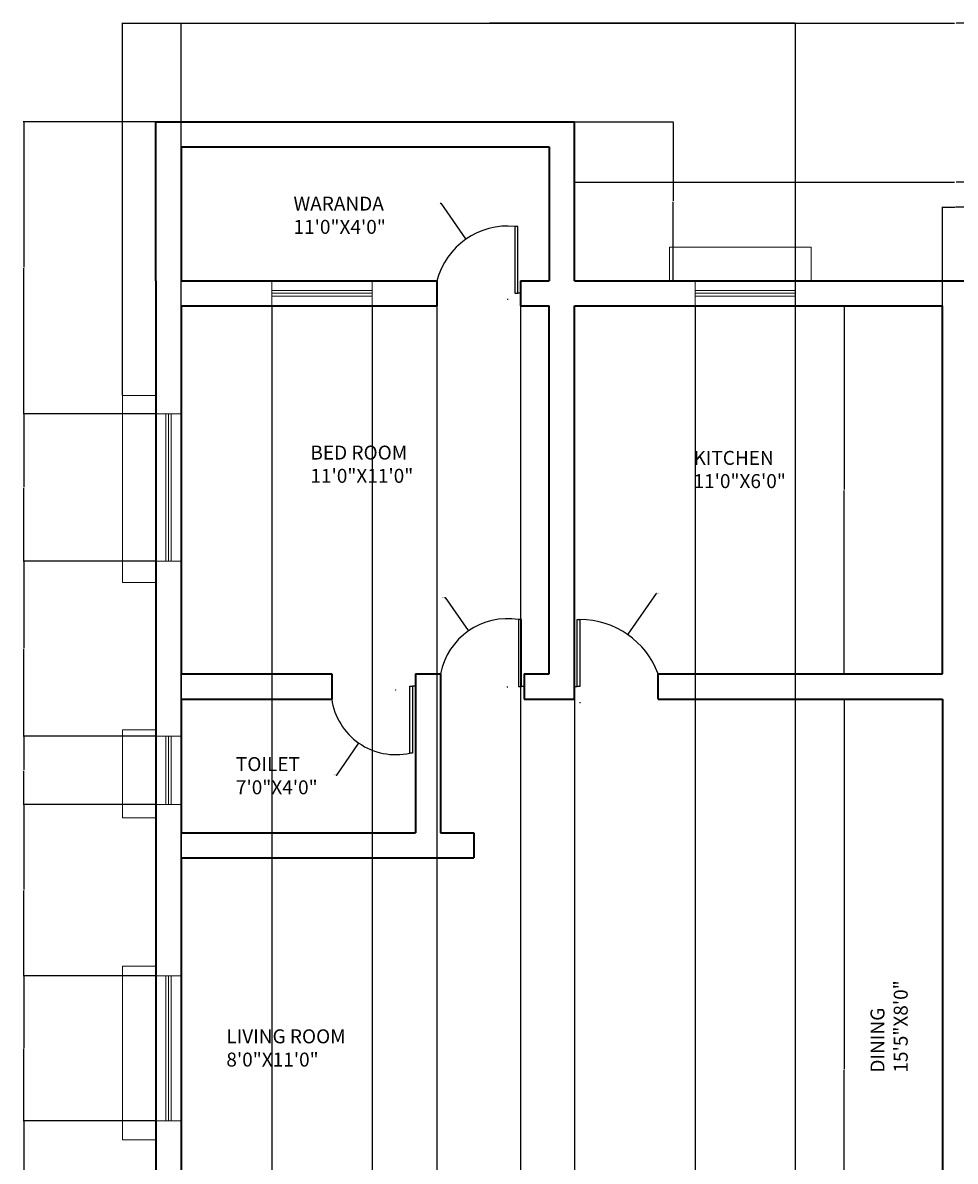
# Model space of a CAD drawing. Units: inches. Extents: x -35 to 633, y -653 to 119.
# Tile 3 of 4: x -35 to 299, y -289 to 119. Entities that reach past the tile are written whole.
import ezdxf

# ---------------------------------------------------------------- set-up
doc = ezdxf.new("R2010")
doc.units = ezdxf.units.IN
doc.header["$MEASUREMENT"] = 0
for name, color, linetype, lineweight in [('A-ANNO-DIMS', 2, 'Continuous', 18), ('A-AREA-IDEN', 7, 'Continuous', 18), ('A-DOOR', 3, 'Continuous', 25), ('A-GLAZ', 4, 'Continuous', 20), ('A-GLAZ-PROJ', 4, 'Continuous', 18), ('A-WALL', 7, 'Continuous', 35)]:
    doc.layers.add(name, color=color, linetype=linetype, lineweight=lineweight)
doc.styles.get("Standard").update_dxf_attribs({"font": 'arial.ttf'})
doc.dimstyles.get("Standard").update_dxf_attribs({"dimtxt": 0.18, "dimasz": 0.18, "dimexe": 0.18, "dimexo": 0.0625, "dimgap": 0.09, "dimtad": 0, "dimtih": 1, "dimtoh": 1, "dimdec": 4, "dimzin": 0, "dimdsep": 46, "dimtxsty": 'Standard', "dimcen": 0.09, "dimadec": 0, "dimazin": 0, "dimtfac": 1, "dimtdec": 4, "dimtofl": 0, "dimtmove": 0, "dimatfit": 3, "dimfxl": 1, "dimtolj": 1, "dimtzin": 0, "dimarcsym": 0})

# ---------------------------------------------------------------- blocks, each defined once
blk = doc.blocks.new('DOOR-LEAF-24IN')
for p, q in [((-1, 24), (-2, 24)), ((-2, 24), (-2, 0)), ((-1, 0), (-1, 24)), ((-2, 0), (-1, 0)), ((0, 0), (-1, 0))]:
    blk.add_line(p, q)
blk = doc.blocks.new('*D11')
at = {"layer": 'A-ANNO-DIMS', "color": 0, "lineweight": -2, "transparency": 16777216}
for p, q in [((0.69, -14.75), (0.69, 118.82)), ((0.87, 118.64), (298.9, 118.64)), ((597.51, 118.64), (299.48, 118.64)), ((597.69, -17.48), (597.69, 118.82))]:
    blk.add_line(p, q, dxfattribs=at)
at = {"layer": 'A-ANNO-DIMS', "color": 0, "transparency": 16777216}
for points in [[(0.87, 118.67), (0.87, 118.61), (0.69, 118.64)], [(597.51, 118.67), (597.51, 118.61), (597.69, 118.64)]]:
    blk.add_solid(points, dxfattribs=at)
at = {"layer": 'Defpoints', "color": 0, "transparency": 16777216}
for p in [(597.69, 118.64), (0.69, -14.81), (597.69, -17.55)]:
    blk.add_point(p, dxfattribs=at)
at = {"layer": 'A-ANNO-DIMS', "color": 0, "transparency": 16777216, "insert": (299.19, 118.64), "char_height": 0.18, "attachment_point": 5}
blk.add_mtext('\\A1;597', dxfattribs=at)
blk = doc.blocks.new('*D12')
at = {"layer": 'A-ANNO-DIMS', "color": 0, "lineweight": -2, "transparency": 16777216}
for p, q in [((162.69, 26.35), (162.69, 61.82)), ((162.87, 61.64), (298.9, 61.64)), ((435.51, 61.64), (299.48, 61.64)), ((435.69, 26.35), (435.69, 61.82))]:
    blk.add_line(p, q, dxfattribs=at)
at = {"layer": 'A-ANNO-DIMS', "color": 0, "transparency": 16777216}
for points in [[(162.87, 61.67), (162.87, 61.61), (162.69, 61.64)], [(435.51, 61.67), (435.51, 61.61), (435.69, 61.64)]]:
    blk.add_solid(points, dxfattribs=at)
at = {"layer": 'Defpoints', "color": 0, "transparency": 16777216}
for p in [(435.69, 61.64), (162.69, 26.29), (435.69, 26.29)]:
    blk.add_point(p, dxfattribs=at)
at = {"layer": 'A-ANNO-DIMS', "color": 0, "transparency": 16777216, "insert": (299.19, 61.64), "char_height": 0.18, "attachment_point": 5}
blk.add_mtext('\\A1;273', dxfattribs=at)
blk = doc.blocks.new('*D13')
at = {"layer": 'A-ANNO-DIMS', "color": 0, "lineweight": -2, "transparency": 16777216}
for p, q in [((162.75, 83.29), (198.22, 83.29)), ((198.04, 83.11), (198.04, 54.97)), ((198.04, 26.47), (198.04, 54.61)), ((162.75, 26.29), (198.22, 26.29))]:
    blk.add_line(p, q, dxfattribs=at)
at = {"layer": 'A-ANNO-DIMS', "color": 0, "transparency": 16777216}
for points in [[(198.01, 83.11), (198.07, 83.11), (198.04, 83.29)], [(198.01, 26.47), (198.07, 26.47), (198.04, 26.29)]]:
    blk.add_solid(points, dxfattribs=at)
at = {"layer": 'Defpoints', "color": 0, "transparency": 16777216}
for p in [(162.69, 83.29), (162.69, 26.29), (198.04, 26.29)]:
    blk.add_point(p, dxfattribs=at)
at = {"layer": 'A-ANNO-DIMS', "color": 0, "transparency": 16777216, "insert": (198.04, 54.79), "char_height": 0.18, "attachment_point": 5}
blk.add_mtext('\\A1;57', dxfattribs=at)
blk = doc.blocks.new('*D14')
at = {"layer": 'A-ANNO-DIMS', "color": 0, "lineweight": -2, "transparency": 16777216}
for p, q in [((21.69, 17.22), (21.69, -652.72)), ((54.19, 17.22), (54.19, -652.72)), ((21.87, -652.54), (37.47, -652.54)), ((54.01, -652.54), (38.4, -652.54))]:
    blk.add_line(p, q, dxfattribs=at)
at = {"layer": 'A-ANNO-DIMS', "color": 0, "transparency": 16777216}
for points in [[(21.87, -652.51), (21.87, -652.57), (21.69, -652.54)], [(54.01, -652.51), (54.01, -652.57), (54.19, -652.54)]]:
    blk.add_solid(points, dxfattribs=at)
at = {"layer": 'Defpoints', "color": 0, "transparency": 16777216}
for p in [(21.69, 17.29), (54.19, 17.29), (54.19, -652.54)]:
    blk.add_point(p, dxfattribs=at)
at = {"layer": 'A-ANNO-DIMS', "color": 0, "transparency": 16777216, "insert": (37.94, -652.54), "char_height": 0.18, "attachment_point": 5}
blk.add_mtext('\\A1;32.496', dxfattribs=at)
blk = doc.blocks.new('*D15')
at = {"layer": 'A-ANNO-DIMS', "color": 0, "lineweight": -2, "transparency": 16777216}
for p, q in [((90.19, 17.22), (90.19, -652.72)), ((113.38, 17.22), (113.38, -652.72)), ((90.37, -652.54), (101.32, -652.54)), ((113.2, -652.54), (102.25, -652.54))]:
    blk.add_line(p, q, dxfattribs=at)
at = {"layer": 'A-ANNO-DIMS', "color": 0, "transparency": 16777216}
for points in [[(90.37, -652.51), (90.37, -652.57), (90.19, -652.54)], [(113.2, -652.51), (113.2, -652.57), (113.38, -652.54)]]:
    blk.add_solid(points, dxfattribs=at)
at = {"layer": 'Defpoints', "color": 0, "transparency": 16777216}
for p in [(90.19, 17.29), (113.38, 17.29), (113.38, -652.54)]:
    blk.add_point(p, dxfattribs=at)
at = {"layer": 'A-ANNO-DIMS', "color": 0, "transparency": 16777216, "insert": (101.78, -652.54), "char_height": 0.18, "attachment_point": 5}
blk.add_mtext('\\A1;23.194', dxfattribs=at)
blk = doc.blocks.new('*D16')
at = {"layer": 'A-ANNO-DIMS', "color": 0, "lineweight": -2, "transparency": 16777216}
for p, q in [((113.38, 17.22), (113.38, -652.72)), ((143.38, 17.22), (143.38, -652.72)), ((113.56, -652.54), (128.16, -652.54)), ((143.2, -652.54), (128.6, -652.54))]:
    blk.add_line(p, q, dxfattribs=at)
at = {"layer": 'A-ANNO-DIMS', "color": 0, "transparency": 16777216}
for points in [[(113.56, -652.51), (113.56, -652.57), (113.38, -652.54)], [(143.2, -652.51), (143.2, -652.57), (143.38, -652.54)]]:
    blk.add_solid(points, dxfattribs=at)
at = {"layer": 'Defpoints', "color": 0, "transparency": 16777216}
for p in [(113.38, 17.29), (143.38, 17.29), (143.38, -652.54)]:
    blk.add_point(p, dxfattribs=at)
at = {"layer": 'A-ANNO-DIMS', "color": 0, "transparency": 16777216, "insert": (128.38, -652.54), "char_height": 0.18, "attachment_point": 5}
blk.add_mtext('\\A1;30', dxfattribs=at)
blk = doc.blocks.new('*D17')
at = {"layer": 'A-ANNO-DIMS', "color": 0, "lineweight": -2, "transparency": 16777216}
for p, q in [((162.69, 17.22), (162.69, -652.72)), ((205.96, 17.22), (205.96, -652.72)), ((162.87, -652.54), (183.93, -652.54)), ((205.78, -652.54), (184.72, -652.54))]:
    blk.add_line(p, q, dxfattribs=at)
at = {"layer": 'A-ANNO-DIMS', "color": 0, "transparency": 16777216}
for points in [[(162.87, -652.51), (162.87, -652.57), (162.69, -652.54)], [(205.78, -652.51), (205.78, -652.57), (205.96, -652.54)]]:
    blk.add_solid(points, dxfattribs=at)
at = {"layer": 'Defpoints', "color": 0, "transparency": 16777216}
for p in [(162.69, 17.29), (205.96, 17.29), (205.96, -652.54)]:
    blk.add_point(p, dxfattribs=at)
at = {"layer": 'A-ANNO-DIMS', "color": 0, "transparency": 16777216, "insert": (184.33, -652.54), "char_height": 0.18, "attachment_point": 5}
blk.add_mtext('\\A1;43.27', dxfattribs=at)
blk = doc.blocks.new('*D18')
at = {"layer": 'A-ANNO-DIMS', "color": 0, "lineweight": -2, "transparency": 16777216}
for p, q in [((294.69, 17.35), (294.69, 52.82)), ((294.87, 52.64), (299.04, 52.64)), ((303.51, 52.64), (299.34, 52.64)), ((303.69, 17.35), (303.69, 52.82))]:
    blk.add_line(p, q, dxfattribs=at)
at = {"layer": 'A-ANNO-DIMS', "color": 0, "transparency": 16777216}
for points in [[(294.87, 52.67), (294.87, 52.61), (294.69, 52.64)], [(303.51, 52.67), (303.51, 52.61), (303.69, 52.64)]]:
    blk.add_solid(points, dxfattribs=at)
at = {"layer": 'Defpoints', "color": 0, "transparency": 16777216}
for p in [(303.69, 52.64), (294.69, 17.29), (303.69, 17.29)]:
    blk.add_point(p, dxfattribs=at)
at = {"layer": 'A-ANNO-DIMS', "color": 0, "transparency": 16777216, "insert": (299.19, 52.64), "char_height": 0.18, "attachment_point": 5}
blk.add_mtext('\\A1;9', dxfattribs=at)
blk = doc.blocks.new('*D25')
at = {"layer": 'A-ANNO-DIMS', "color": 0, "lineweight": -2, "transparency": 16777216}
for p, q in [((12.63, 83.29), (-34.84, 83.29)), ((-34.66, 83.11), (-34.66, 31.12)), ((-34.66, -21.23), (-34.66, 30.76)), ((12.63, -21.41), (-34.84, -21.41))]:
    blk.add_line(p, q, dxfattribs=at)
at = {"layer": 'A-ANNO-DIMS', "color": 0, "transparency": 16777216}
for points in [[(-34.69, 83.11), (-34.63, 83.11), (-34.66, 83.29)], [(-34.69, -21.23), (-34.63, -21.23), (-34.66, -21.41)]]:
    blk.add_solid(points, dxfattribs=at)
at = {"layer": 'Defpoints', "color": 0, "transparency": 16777216}
for p in [(12.69, 83.29), (-34.66, -21.41), (12.69, -21.41)]:
    blk.add_point(p, dxfattribs=at)
at = {"layer": 'A-ANNO-DIMS', "color": 0, "transparency": 16777216, "insert": (-34.66, 30.94), "char_height": 0.18, "attachment_point": 5}
blk.add_mtext('\\A1;104.7', dxfattribs=at)
blk = doc.blocks.new('*D26')
at = {"layer": 'A-ANNO-DIMS', "color": 0, "lineweight": -2, "transparency": 16777216}
for p, q in [((12.63, -21.41), (-34.84, -21.41)), ((-34.66, -21.59), (-34.66, -47.65)), ((-34.66, -74.08), (-34.66, -48.02)), ((12.63, -74.26), (-34.84, -74.26))]:
    blk.add_line(p, q, dxfattribs=at)
at = {"layer": 'A-ANNO-DIMS', "color": 0, "transparency": 16777216}
for points in [[(-34.69, -21.59), (-34.63, -21.59), (-34.66, -21.41)], [(-34.69, -74.08), (-34.63, -74.08), (-34.66, -74.26)]]:
    blk.add_solid(points, dxfattribs=at)
at = {"layer": 'Defpoints', "color": 0, "transparency": 16777216}
for p in [(12.69, -21.41), (-34.66, -74.26), (12.69, -74.26)]:
    blk.add_point(p, dxfattribs=at)
at = {"layer": 'A-ANNO-DIMS', "color": 0, "transparency": 16777216, "insert": (-34.66, -47.84), "char_height": 0.18, "attachment_point": 5}
blk.add_mtext('\\A1;52.85', dxfattribs=at)
blk = doc.blocks.new('*D27')
at = {"layer": 'A-ANNO-DIMS', "color": 0, "lineweight": -2, "transparency": 16777216}
for p, q in [((12.63, -74.26), (-34.84, -74.26)), ((-34.66, -74.44), (-34.66, -105.47)), ((-34.66, -136.87), (-34.66, -105.84)), ((12.63, -137.05), (-34.84, -137.05))]:
    blk.add_line(p, q, dxfattribs=at)
at = {"layer": 'A-ANNO-DIMS', "color": 0, "transparency": 16777216}
for points in [[(-34.69, -74.44), (-34.63, -74.44), (-34.66, -74.26)], [(-34.69, -136.87), (-34.63, -136.87), (-34.66, -137.05)]]:
    blk.add_solid(points, dxfattribs=at)
at = {"layer": 'Defpoints', "color": 0, "transparency": 16777216}
for p in [(12.69, -74.26), (-34.66, -137.05), (12.69, -137.05)]:
    blk.add_point(p, dxfattribs=at)
at = {"layer": 'A-ANNO-DIMS', "color": 0, "transparency": 16777216, "insert": (-34.66, -105.66), "char_height": 0.18, "attachment_point": 5}
blk.add_mtext('\\A1;62.79', dxfattribs=at)
blk = doc.blocks.new('*D28')
at = {"layer": 'A-ANNO-DIMS', "color": 0, "lineweight": -2, "transparency": 16777216}
for p, q in [((12.63, -137.05), (-34.84, -137.05)), ((-34.66, -137.23), (-34.66, -149.1)), ((-34.66, -161.33), (-34.66, -149.46)), ((12.63, -161.51), (-34.84, -161.51))]:
    blk.add_line(p, q, dxfattribs=at)
at = {"layer": 'A-ANNO-DIMS', "color": 0, "transparency": 16777216}
for points in [[(-34.69, -137.23), (-34.63, -137.23), (-34.66, -137.05)], [(-34.69, -161.33), (-34.63, -161.33), (-34.66, -161.51)]]:
    blk.add_solid(points, dxfattribs=at)
at = {"layer": 'Defpoints', "color": 0, "transparency": 16777216}
for p in [(12.69, -137.05), (-34.66, -161.51), (12.69, -161.51)]:
    blk.add_point(p, dxfattribs=at)
at = {"layer": 'A-ANNO-DIMS', "color": 0, "transparency": 16777216, "insert": (-34.66, -149.28), "char_height": 0.18, "attachment_point": 5}
blk.add_mtext('\\A1;24.463', dxfattribs=at)
blk = doc.blocks.new('*D29')
at = {"layer": 'A-ANNO-DIMS', "color": 0, "lineweight": -2, "transparency": 16777216}
for p, q in [((12.63, -161.51), (-34.84, -161.51)), ((-34.66, -161.69), (-34.66, -192.06)), ((-34.66, -222.79), (-34.66, -192.43)), ((12.63, -222.97), (-34.84, -222.97))]:
    blk.add_line(p, q, dxfattribs=at)
at = {"layer": 'A-ANNO-DIMS', "color": 0, "transparency": 16777216}
for points in [[(-34.69, -161.69), (-34.63, -161.69), (-34.66, -161.51)], [(-34.69, -222.79), (-34.63, -222.79), (-34.66, -222.97)]]:
    blk.add_solid(points, dxfattribs=at)
at = {"layer": 'Defpoints', "color": 0, "transparency": 16777216}
for p in [(12.69, -161.51), (-34.66, -222.97), (12.69, -222.97)]:
    blk.add_point(p, dxfattribs=at)
at = {"layer": 'A-ANNO-DIMS', "color": 0, "transparency": 16777216, "insert": (-34.66, -192.24), "char_height": 0.18, "attachment_point": 5}
blk.add_mtext('\\A1;61.46', dxfattribs=at)
blk = doc.blocks.new('*D30')
at = {"layer": 'A-ANNO-DIMS', "color": 0, "lineweight": -2, "transparency": 16777216}
for p, q in [((12.63, -222.97), (-34.84, -222.97)), ((-34.66, -223.15), (-34.66, -248.78)), ((-34.66, -274.78), (-34.66, -249.15)), ((12.63, -274.96), (-34.84, -274.96))]:
    blk.add_line(p, q, dxfattribs=at)
at = {"layer": 'A-ANNO-DIMS', "color": 0, "transparency": 16777216}
for points in [[(-34.69, -223.15), (-34.63, -223.15), (-34.66, -222.97)], [(-34.69, -274.78), (-34.63, -274.78), (-34.66, -274.96)]]:
    blk.add_solid(points, dxfattribs=at)
at = {"layer": 'Defpoints', "color": 0, "transparency": 16777216}
for p in [(12.69, -222.97), (-34.66, -274.96), (12.69, -274.96)]:
    blk.add_point(p, dxfattribs=at)
at = {"layer": 'A-ANNO-DIMS', "color": 0, "transparency": 16777216, "insert": (-34.66, -248.97), "char_height": 0.18, "attachment_point": 5}
blk.add_mtext('\\A1;51.99', dxfattribs=at)
blk = doc.blocks.new('*D31')
at = {"layer": 'A-ANNO-DIMS', "color": 0, "lineweight": -2, "transparency": 16777216}
for p, q in [((12.63, -274.96), (-34.84, -274.96)), ((-34.66, -275.14), (-34.66, -304.9)), ((-34.66, -335.03), (-34.66, -305.27)), ((12.63, -335.21), (-34.84, -335.21))]:
    blk.add_line(p, q, dxfattribs=at)
at = {"layer": 'A-ANNO-DIMS', "color": 0, "transparency": 16777216}
for points in [[(-34.69, -275.14), (-34.63, -275.14), (-34.66, -274.96)], [(-34.69, -335.03), (-34.63, -335.03), (-34.66, -335.21)]]:
    blk.add_solid(points, dxfattribs=at)
at = {"layer": 'Defpoints', "color": 0, "transparency": 16777216}
for p in [(12.69, -274.96), (-34.66, -335.21), (12.69, -335.21)]:
    blk.add_point(p, dxfattribs=at)
at = {"layer": 'A-ANNO-DIMS', "color": 0, "transparency": 16777216, "insert": (-34.66, -305.09), "char_height": 0.18, "attachment_point": 5}
blk.add_mtext('\\A1;60.25', dxfattribs=at)
blk = doc.blocks.new('*D36')
at = {"layer": 'A-ANNO-DIMS', "color": 0, "lineweight": -2, "transparency": 16777216}
for p, q in [((21.69, -546.65), (21.69, 118.82)), ((21.87, 118.64), (131.44, 118.64)), ((241.8, 118.64), (132.23, 118.64)), ((241.98, -546.65), (241.98, 118.82))]:
    blk.add_line(p, q, dxfattribs=at)
at = {"layer": 'A-ANNO-DIMS', "color": 0, "transparency": 16777216}
for points in [[(21.87, 118.67), (21.87, 118.61), (21.69, 118.64)], [(241.8, 118.67), (241.8, 118.61), (241.98, 118.64)]]:
    blk.add_solid(points, dxfattribs=at)
at = {"layer": 'Defpoints', "color": 0, "transparency": 16777216}
for p in [(241.98, 118.64), (21.69, -546.71), (241.98, -546.71)]:
    blk.add_point(p, dxfattribs=at)
at = {"layer": 'A-ANNO-DIMS', "color": 0, "transparency": 16777216, "insert": (131.83, 118.64), "char_height": 0.18, "attachment_point": 5}
blk.add_mtext('\\A1;220.3', dxfattribs=at)
blk = doc.blocks.new('*D38')
at = {"layer": 'A-ANNO-DIMS', "color": 0, "lineweight": -2, "transparency": 16777216}
for p, q in [((294.63, 17.29), (259.16, 17.29)), ((259.34, 17.11), (259.34, -48.53)), ((259.34, -114.53), (259.34, -48.89)), ((294.63, -114.71), (259.16, -114.71))]:
    blk.add_line(p, q, dxfattribs=at)
at = {"layer": 'A-ANNO-DIMS', "color": 0, "transparency": 16777216}
for points in [[(259.31, 17.11), (259.37, 17.11), (259.34, 17.29)], [(259.31, -114.53), (259.37, -114.53), (259.34, -114.71)]]:
    blk.add_solid(points, dxfattribs=at)
at = {"layer": 'Defpoints', "color": 0, "transparency": 16777216}
for p in [(259.34, 17.29), (294.69, 17.29), (294.69, -114.71)]:
    blk.add_point(p, dxfattribs=at)
at = {"layer": 'A-ANNO-DIMS', "color": 0, "transparency": 16777216, "insert": (259.34, -48.71), "char_height": 0.18, "attachment_point": 5}
blk.add_mtext('\\A1;132', dxfattribs=at)
blk = doc.blocks.new('*D46')
at = {"layer": 'A-ANNO-DIMS', "color": 0, "lineweight": -2, "transparency": 16777216}
for p, q in [((294.63, -123.71), (259.16, -123.71)), ((259.34, -123.89), (259.34, -256.48)), ((259.34, -389.42), (259.34, -256.84)), ((294.63, -389.6), (259.16, -389.6))]:
    blk.add_line(p, q, dxfattribs=at)
at = {"layer": 'A-ANNO-DIMS', "color": 0, "transparency": 16777216}
for points in [[(259.31, -123.89), (259.37, -123.89), (259.34, -123.71)], [(259.31, -389.42), (259.37, -389.42), (259.34, -389.6)]]:
    blk.add_solid(points, dxfattribs=at)
at = {"layer": 'Defpoints', "color": 0, "transparency": 16777216}
for p in [(259.34, -123.71), (294.69, -123.71), (294.69, -389.6)]:
    blk.add_point(p, dxfattribs=at)
at = {"layer": 'A-ANNO-DIMS', "color": 0, "transparency": 16777216, "insert": (259.34, -256.66), "char_height": 0.18, "attachment_point": 5}
blk.add_mtext('\\A1;265.9', dxfattribs=at)
blk = doc.blocks.new('*D47')
at = {"layer": 'A-ANNO-DIMS', "color": 0, "lineweight": -2, "transparency": 16777216}
for p, q in [((294.69, -123.78), (294.69, -652.72)), ((126.69, -312.78), (126.69, -652.72)), ((126.87, -652.54), (210.41, -652.54)), ((294.51, -652.54), (210.97, -652.54))]:
    blk.add_line(p, q, dxfattribs=at)
at = {"layer": 'A-ANNO-DIMS', "color": 0, "transparency": 16777216}
for points in [[(126.87, -652.51), (126.87, -652.57), (126.69, -652.54)], [(294.51, -652.51), (294.51, -652.57), (294.69, -652.54)]]:
    blk.add_solid(points, dxfattribs=at)
at = {"layer": 'Defpoints', "color": 0, "transparency": 16777216}
for p in [(294.69, -123.71), (126.69, -312.71), (294.69, -652.54)]:
    blk.add_point(p, dxfattribs=at)
at = {"layer": 'A-ANNO-DIMS', "color": 0, "transparency": 16777216, "insert": (210.69, -652.54), "char_height": 0.18, "attachment_point": 5}
blk.add_mtext('\\A1;168', dxfattribs=at)
blk = doc.blocks.new('*D52')
at = {"layer": 'A-ANNO-DIMS', "color": 0, "lineweight": -2, "transparency": 16777216}
for p, q in [((191.97, -85.9), (181.87, -100.4)), ((192.15, -85.9), (191.97, -85.9)), ((164.66, -124.97), (164.84, -124.97)), ((164.75, -125.06), (164.75, -124.88))]:
    blk.add_line(p, q, dxfattribs=at)
at = {"layer": 'A-ANNO-DIMS', "color": 0, "transparency": 16777216}
blk.add_solid([(181.84, -100.39), (181.89, -100.42), (181.76, -100.55)], dxfattribs=at)
at = {"layer": 'Defpoints', "color": 0, "transparency": 16777216}
for p in [(181.76, -100.55), (164.75, -124.97)]:
    blk.add_point(p, dxfattribs=at)
at = {"layer": 'A-ANNO-DIMS', "color": 0, "transparency": 16777216, "insert": (192.63, -85.9), "char_height": 0.18, "attachment_point": 5}
blk.add_mtext('\\A1;R29.76', dxfattribs=at)
blk = doc.blocks.new('*D55')
at = {"layer": 'A-ANNO-DIMS', "color": 0, "lineweight": -2, "transparency": 16777216}
for p, q in [((114.6, 54.14), (114.78, 54.14)), ((114.78, 54.14), (123.68, 41.35)), ((138.71, 19.65), (138.89, 19.65)), ((138.8, 19.56), (138.8, 19.74))]:
    blk.add_line(p, q, dxfattribs=at)
at = {"layer": 'A-ANNO-DIMS', "color": 0, "transparency": 16777216}
blk.add_solid([(123.7, 41.37), (123.66, 41.33), (123.78, 41.2)], dxfattribs=at)
at = {"layer": 'Defpoints', "color": 0, "transparency": 16777216}
for p in [(123.78, 41.2), (138.8, 19.65)]:
    blk.add_point(p, dxfattribs=at)
at = {"layer": 'A-ANNO-DIMS', "color": 0, "transparency": 16777216, "insert": (114.12, 54.14), "char_height": 0.18, "attachment_point": 5}
blk.add_mtext('\\A1;R26.27', dxfattribs=at)
blk = doc.blocks.new('*D60')
at = {"layer": 'A-ANNO-DIMS', "color": 0, "lineweight": -2, "transparency": 16777216}
for p, q in [((116.16, -87.24), (116.34, -87.24)), ((116.34, -87.24), (124.62, -99.12)), ((138.6, -119.32), (138.78, -119.32)), ((138.69, -119.41), (138.69, -119.23))]:
    blk.add_line(p, q, dxfattribs=at)
at = {"layer": 'A-ANNO-DIMS', "color": 0, "transparency": 16777216}
blk.add_solid([(124.64, -99.1), (124.6, -99.14), (124.72, -99.27)], dxfattribs=at)
at = {"layer": 'Defpoints', "color": 0, "transparency": 16777216}
for p in [(124.72, -99.27), (138.69, -119.32)]:
    blk.add_point(p, dxfattribs=at)
at = {"layer": 'A-ANNO-DIMS', "color": 0, "transparency": 16777216, "insert": (115.61, -87.24), "char_height": 0.18, "attachment_point": 5}
blk.add_mtext('\\A1;R24.433', dxfattribs=at)
blk = doc.blocks.new('*D61')
at = {"layer": 'A-ANNO-DIMS', "color": 0, "lineweight": -2, "transparency": 16777216}
for p, q in [((98.56, -120.47), (98.74, -120.47)), ((98.65, -120.56), (98.65, -120.38)), ((77.53, -150.97), (85.35, -139.68)), ((77.35, -150.97), (77.53, -150.97))]:
    blk.add_line(p, q, dxfattribs=at)
at = {"layer": 'A-ANNO-DIMS', "color": 0, "transparency": 16777216}
blk.add_solid([(85.32, -139.66), (85.37, -139.7), (85.45, -139.53)], dxfattribs=at)
at = {"layer": 'Defpoints', "color": 0, "transparency": 16777216}
for p in [(98.65, -120.47), (85.45, -139.53)]:
    blk.add_point(p, dxfattribs=at)
at = {"layer": 'A-ANNO-DIMS', "color": 0, "transparency": 16777216, "insert": (76.87, -150.97), "char_height": 0.18, "attachment_point": 5}
blk.add_mtext('\\A1;R23.19', dxfattribs=at)

msp = doc.modelspace()

# ---------------------------------------------------------------- linework, layer by layer
at = {"layer": 'A-DOOR'}
for centre, radius, start, end in [((138.7952, 19.6465), 26.268, 84.352041, 165.35687), ((138.6865, -119.316), 24.4333, 80.567749, 169.141162), ((164.7548, -124.9734), 29.7605, 20.167594, 90.123495), ((98.6518, -120.4692), 23.1891, 188.041001, 282.550097)]:
    msp.add_arc(centre, radius, start, end, dxfattribs=at)
at = {"layer": 'A-GLAZ'}
for p, q in [((54.1862, 26.287), (54.1862, 17.287)), ((90.1862, 26.287), (90.1862, 17.287)), ((54.1862, 22.787), (90.1862, 22.787)), ((54.1862, 21.787), (90.1862, 21.787)), ((54.1862, 20.787), (90.1862, 20.787)), ((206.5892, 22.787), (205.9605, 22.787)), ((206.5892, 21.787), (205.9605, 21.787)), ((206.5892, 20.787), (205.9605, 20.787)), ((206.5892, 22.787), (241.9605, 22.787)), ((206.5892, 21.787), (241.9605, 21.787)), ((206.5892, 20.787), (241.9605, 20.787)), ((12.6907, -21.4113), (21.6907, -21.4113)), ((16.1907, -21.4113), (16.1907, -74.2608)), ((17.1907, -21.4113), (17.1907, -74.2608)), ((18.1907, -21.4113), (18.1907, -74.2608)), ((12.6907, -74.2608), (21.6907, -74.2608)), ((12.6907, -137.0511), (21.6907, -137.0511)), ((16.1907, -137.0511), (16.1907, -161.5138)), ((17.1907, -137.0511), (17.1907, -161.5138)), ((18.1907, -137.0511), (18.1907, -161.5138)), ((12.6907, -161.5138), (21.6907, -161.5138)), ((12.6907, -222.9733), (21.6907, -222.9733)), ((16.1907, -222.9733), (16.1907, -274.9586)), ((17.1907, -222.9733), (17.1907, -274.9586)), ((18.1907, -222.9733), (18.1907, -274.9586)), ((12.6907, -274.9586), (21.6907, -274.9586))]:
    msp.add_line(p, q, dxfattribs=at)
msp.add_lwpolyline([(205.9605, 26.287), (241.9605, 26.287), (241.9605, 17.287), (205.9605, 17.287)], close=True, dxfattribs=at)
at = {"layer": 'A-GLAZ-PROJ'}
for p, q in [((196.8039, 26.287), (196.8039, 38.287)), ((196.8039, 38.287), (247.5262, 38.287)), ((247.5262, 38.287), (247.5262, 26.287)), ((12.6907, -14.8086), (0.6907, -14.8086)), ((0.6907, -14.8086), (0.6907, -81.9128)), ((0.6907, -81.9128), (12.6907, -81.9128)), ((12.6907, -134.7073), (0.6907, -134.7073)), ((0.6907, -134.7073), (0.6907, -166.3523)), ((0.6907, -166.3523), (12.6907, -166.3523)), ((12.6907, -219.5127), (0.6907, -219.5127)), ((0.6907, -219.5127), (0.6907, -281.7548)), ((0.6907, -281.7548), (12.6907, -281.7548))]:
    msp.add_line(p, q, dxfattribs=at)
at = {"layer": 'A-WALL'}
for p, q in [((12.6907, 26.287), (12.6907, 83.287)), ((12.6907, 83.287), (21.6907, 83.287)), ((21.6907, 83.287), (162.6907, 83.287)), ((162.6907, 26.287), (162.6907, 83.287)), ((21.6907, 74.287), (153.6907, 74.287)), ((21.6907, 74.287), (21.6907, 26.287)), ((153.6907, 74.287), (153.6907, 26.287)), ((12.6907, 26.287), (12.6907, 17.287)), ((21.6907, 26.287), (113.3804, 26.287)), ((113.3804, 26.287), (113.3804, 17.287)), ((143.3804, 26.287), (143.3804, 17.287)), ((143.3804, 26.287), (153.6907, 26.287)), ((162.6907, 26.287), (435.6907, 26.287)), ((12.6907, 17.287), (12.6907, -114.713)), ((21.6907, 17.287), (113.3804, 17.287)), ((21.6907, 17.287), (21.6907, -114.713)), ((143.3804, 17.287), (153.6907, 17.287)), ((153.6907, -114.713), (153.6907, 17.287)), ((162.6907, -114.713), (162.6907, 17.287)), ((162.6907, 17.287), (294.6907, 17.287)), ((294.6907, -114.713), (294.6907, 17.287)), ((12.6907, -114.713), (12.6907, -555.713)), ((21.6907, -114.713), (75.6907, -114.713)), ((75.6907, -114.713), (75.6907, -123.713)), ((105.6907, -114.713), (105.6907, -171.713)), ((105.6907, -114.713), (114.6907, -114.713)), ((114.6907, -114.713), (114.6907, -171.713)), ((144.6907, -114.713), (144.6907, -123.713)), ((144.6907, -114.713), (153.6907, -114.713)), ((162.6907, -123.713), (162.6907, -114.713)), ((192.6907, -123.713), (192.6907, -114.713)), ((192.6907, -114.713), (294.6907, -114.713)), ((21.6907, -123.713), (75.6907, -123.713)), ((21.6907, -123.713), (21.6907, -171.713)), ((144.6907, -123.713), (153.6907, -123.713)), ((153.6907, -123.713), (162.6907, -123.713)), ((192.6907, -123.713), (294.6907, -123.713)), ((294.6907, -123.713), (294.6907, -389.6034)), ((21.6907, -171.713), (105.6907, -171.713)), ((114.6907, -171.713), (126.6907, -171.713)), ((126.6907, -171.713), (126.6907, -180.713)), ((21.6907, -180.713), (114.6907, -180.713)), ((21.6907, -180.713), (21.6907, -312.713)), ((114.6907, -180.713), (126.6907, -180.713))]:
    msp.add_line(p, q, dxfattribs=at)

# ---------------------------------------------------------------- block references
at = {"layer": 'A-DOOR'}
for p in [(143.3804, 21.787), (144.6907, -119.213)]:
    msp.add_blockref('DOOR-LEAF-24IN', p, dxfattribs=at)
at = {"layer": 'A-DOOR', "extrusion": (0, 0, -1), "zscale": -1}
msp.add_blockref('DOOR-LEAF-24IN', (-162.6907, -119.213), dxfattribs=at)
at = {"layer": 'A-DOOR', "extrusion": (0, 0, -1), "zscale": -1, "rotation": 180}
msp.add_blockref('DOOR-LEAF-24IN', (-105.6907, -119.1043), dxfattribs=at)

# ---------------------------------------------------------------- texts
at = {"layer": 'A-AREA-IDEN', "char_height": 5, "attachment_point": 1}
for s, width, insert in [('WARANDA\\P11\'0"X4\'0"', 24.624866, (62.0025, 56.4574)), ('BED ROOM\\P11\'0"X11\'0"', 64.884056, (68.0565, -32.8336)), ('KITCHEN\\P11\'0"X6\'0"', 40.946262, (205.3839, -34.7212)), ('TOILET\\P7\'0"X4\'0"', 26.587234, (41.3511, -144.5352)), ('LIVING ROOM\\P8\'0"X11\'0"', 66.509643, (37.9281, -242.1824))]:
    msp.add_mtext_dynamic_manual_height_columns(s, width=width, gutter_width=25, heights=[0], dxfattribs=dict(at, insert=insert))
at = {"layer": 'A-AREA-IDEN', "insert": (268.8293, -257.6812), "char_height": 5, "attachment_point": 1, "rotation": 90}
msp.add_mtext_dynamic_manual_height_columns('DINING\\P15\'5"X8\'0"', width=68.431972, gutter_width=25, heights=[0], dxfattribs=at)

# ---------------------------------------------------------------- dimensions: what is measured, and where the dimension line sits
at = {"layer": 'A-ANNO-DIMS'}
for base, p1, p2, override, picture, middle in [((597.6907, 118.637), (0.6907, -14.8086), (597.6907, -17.5469), {"dimdec": 0, "dimlfac": 1, "dimrnd": 0, "dimzin": 0, "dimdsep": 46, "dimlunit": 2}, '*D11', (299.1907, 118.637)), ((241.9768, 118.637), (21.6907, -546.713), (241.9768, -546.713), {"dimdec": 1, "dimlfac": 1, "dimrnd": 0, "dimzin": 0, "dimdsep": 46, "dimlunit": 2}, '*D36', (131.8337, 118.637)), ((435.6907, 61.637), (162.6907, 26.287), (435.6907, 26.287), {"dimdec": 0, "dimlfac": 1, "dimrnd": 0, "dimzin": 0, "dimdsep": 46, "dimlunit": 2}, '*D12', (299.1907, 61.637)), ((303.6907, 52.637), (294.6907, 17.287), (303.6907, 17.287), {"dimdec": 0, "dimlfac": 1, "dimrnd": 0, "dimzin": 0, "dimdsep": 46, "dimlunit": 2}, '*D18', (299.1907, 52.637)), ((54.18621, -652.537), (21.69066, 17.28704), (54.18621, 17.28704), {"dimdec": 3, "dimlfac": 1, "dimrnd": 0, "dimzin": 0, "dimdsep": 46, "dimlunit": 2}, '*D14', (37.93843, -652.537)), ((113.3804, -652.537), (90.1862, 17.287), (113.3804, 17.287), {"dimdec": 3, "dimlfac": 1, "dimrnd": 0, "dimzin": 0, "dimdsep": 46, "dimlunit": 2}, '*D15', (101.7833, -652.537)), ((143.3804, -652.537), (113.3804, 17.287), (143.3804, 17.287), {"dimdec": 0, "dimlfac": 1, "dimrnd": 0, "dimzin": 0, "dimdsep": 46, "dimlunit": 2}, '*D16', (128.3804, -652.537)), ((205.9605, -652.537), (162.6907, 17.287), (205.9605, 17.287), {"dimdec": 2, "dimlfac": 1, "dimrnd": 0, "dimzin": 0, "dimdsep": 46, "dimlunit": 2}, '*D17', (184.3256, -652.537)), ((294.6907, -652.537), (126.6907, -312.713), (294.6907, -123.713), {"dimdec": 0, "dimlfac": 1, "dimrnd": 0, "dimzin": 0, "dimdsep": 46, "dimlunit": 2}, '*D47', (210.6907, -652.537))]:
    dim = msp.add_linear_dim(base=base, p1=p1, p2=p2, dimstyle='Standard', override=override, dxfattribs=at)
    dim.commit()
    dim.dimension.update_dxf_attribs({"geometry": picture, "text_midpoint": middle})
for base, p1, p2, angle, override, picture, middle in [((-34.6593, -21.4113), (12.6907, 83.287), (12.6907, -21.4113), 90, {"dimdec": 1, "dimlfac": 1, "dimrnd": 0, "dimzin": 0, "dimdsep": 46, "dimlunit": 2}, '*D25', (-34.6593, 30.9379)), ((198.0407, 26.287), (162.6907, 83.287), (162.6907, 26.287), 270, {"dimdec": 0, "dimlfac": 1, "dimrnd": 0, "dimzin": 0, "dimdsep": 46, "dimlunit": 2}, '*D13', (198.0407, 54.787)), ((259.3407, 17.287), (294.6907, -114.713), (294.6907, 17.287), 90, {"dimdec": 0, "dimlfac": 1, "dimrnd": 0, "dimzin": 0, "dimdsep": 46, "dimlunit": 2}, '*D38', (259.3407, -48.713)), ((-34.6593, -74.2608), (12.6907, -21.4113), (12.6907, -74.2608), 90, {"dimdec": 2, "dimlfac": 1, "dimrnd": 0, "dimzin": 0, "dimdsep": 46, "dimlunit": 2}, '*D26', (-34.6593, -47.8361)), ((-34.6593, -137.0511), (12.6907, -74.2608), (12.6907, -137.0511), 90, {"dimdec": 2, "dimlfac": 1, "dimrnd": 0, "dimzin": 0, "dimdsep": 46, "dimlunit": 2}, '*D27', (-34.6593, -105.6559)), ((259.3407, -123.713), (294.6907, -389.6034), (294.6907, -123.713), 90, {"dimdec": 1, "dimlfac": 1, "dimrnd": 0, "dimzin": 0, "dimdsep": 46, "dimlunit": 2}, '*D46', (259.3407, -256.6582)), ((-34.6593, -161.5138), (12.6907, -137.0511), (12.6907, -161.5138), 90, {"dimdec": 3, "dimlfac": 1, "dimrnd": 0, "dimzin": 0, "dimdsep": 46, "dimlunit": 2}, '*D28', (-34.6593, -149.2824)), ((-34.6593, -222.9733), (12.6907, -161.5138), (12.6907, -222.9733), 90, {"dimdec": 2, "dimlfac": 1, "dimrnd": 0, "dimzin": 0, "dimdsep": 46, "dimlunit": 2}, '*D29', (-34.6593, -192.2435)), ((-34.6593, -274.9586), (12.6907, -222.9733), (12.6907, -274.9586), 90, {"dimdec": 2, "dimlfac": 1, "dimrnd": 0, "dimzin": 0, "dimdsep": 46, "dimlunit": 2}, '*D30', (-34.6593, -248.966)), ((-34.6593, -335.213), (12.6907, -274.9586), (12.6907, -335.213), 90, {"dimdec": 2, "dimlfac": 1, "dimrnd": 0, "dimzin": 0, "dimdsep": 46, "dimlunit": 2}, '*D31', (-34.6593, -305.0858))]:
    dim = msp.add_linear_dim(base=base, p1=p1, p2=p2, angle=angle, dimstyle='Standard', override=override, dxfattribs=at)
    dim.commit()
    dim.dimension.update_dxf_attribs({"geometry": picture, "text_midpoint": middle})
for center, mpoint, override, picture, middle in [((138.7952, 19.6465), (123.7829, 41.2021), {"dimdec": 2, "dimlfac": 1, "dimrnd": 0, "dimzin": 0, "dimdsep": 46, "dimlunit": 2}, '*D55', (114.1158, 54.1354)), ((138.6865, -119.316), (124.7229, -99.2659), {"dimdec": 3, "dimlfac": 1, "dimrnd": 0, "dimzin": 0, "dimdsep": 46, "dimlunit": 2}, '*D60', (115.615, -87.2358)), ((164.7548, -124.9734), (181.763, -100.5519), {"dimdec": 2, "dimlfac": 1, "dimrnd": 0, "dimzin": 0, "dimdsep": 46, "dimlunit": 2}, '*D52', (192.6278, -85.899)), ((98.6518, -120.4692), (85.4491, -139.5329), {"dimdec": 2, "dimlfac": 1, "dimrnd": 0, "dimzin": 0, "dimdsep": 46, "dimlunit": 2}, '*D61', (76.8674, -150.9711))]:
    dim = msp.add_radius_dim(center=center, mpoint=mpoint, dimstyle='Standard', override=override, dxfattribs=at)
    dim.commit()
    dim.dimension.update_dxf_attribs({"geometry": picture, "text_midpoint": middle, "dimtype": 164})

doc.saveas('drawing.dxf')
